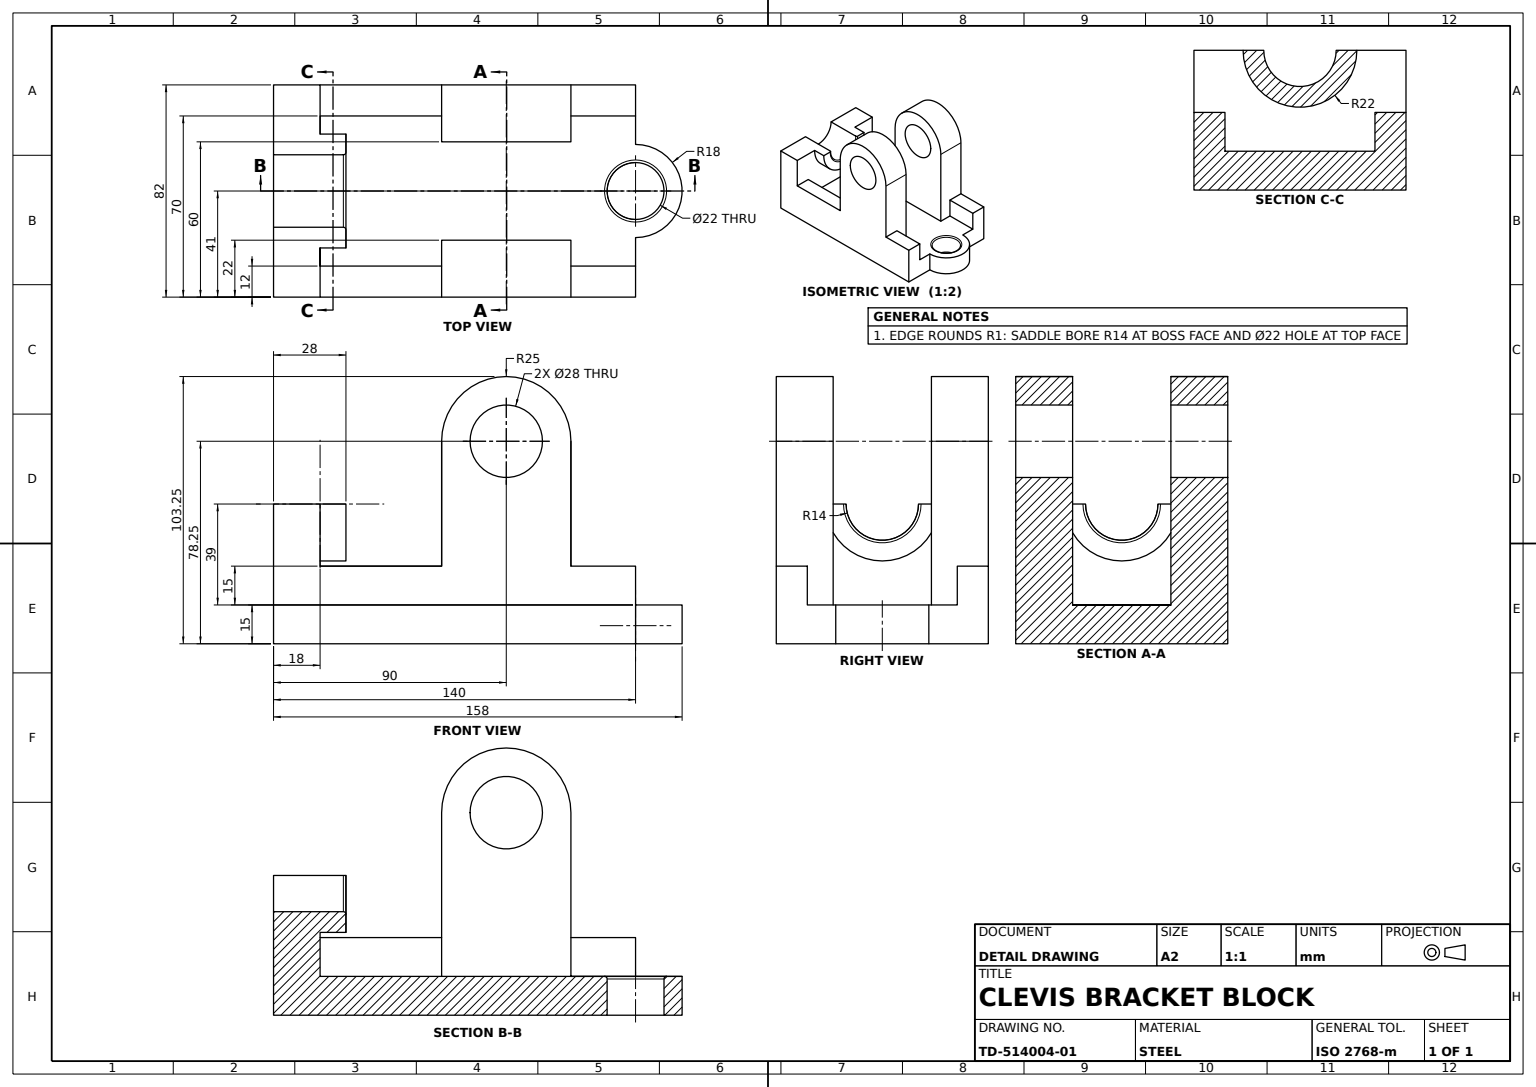
from build123d import *

# Parameters (mm, degrees)
BASE_PLATE_SKETCH_R     = 11
BASE_PLATE_DEPTH        = 15
REAR_WALL_SKETCH_W      = 18
REAR_WALL_SKETCH_H      = 82
REAR_WALL_DEPTH         = 39
STEP_BLOCKS_SKETCH_W    = 122
STEP_BLOCKS_SKETCH_H    = 12
STEP_BLOCKS_DEPTH       = 15
BEARING_EAR_1_SKETCH_R  = 14
BEARING_EAR_1_DEPTH     = 22
BEARING_START           = -22
BEARING_EAR_2_SKETCH_R  = 14
BEARING_EAR_2_DEPTH     = 22
SADDLE_CUT_DEPTH        = 22
SADDLE_BOSS_DEPTH       = 28
SADDLE_BOSS_FILLET_R1_R = 1
BASE_EDGE_FILLET_R1_R   = 1


with BuildPart() as part:
    # Base Plate Sketch → Base Plate (new body)
    with BuildSketch(Plane(origin=(0, 0, 0), x_dir=(1, 0, 0), z_dir=(0, 1, 0))):
        with BuildLine():
            Line((70, -18), (70, -41))
            Line((70, -41), (-70, -41))
            Line((-70, -41), (-70, 41))
            Line((-70, 41), (70, 41))
            Line((70, 41), (70, 18))
            ThreePointArc((70, 18), (88, 0), (70, -18))
        make_face()
        with Locations(Location((70, 0, 0), (0, 0, 270))):
            Circle(BASE_PLATE_SKETCH_R, mode=Mode.SUBTRACT)
    extrude(amount=BASE_PLATE_DEPTH)

    # Rear Wall Sketch → Rear Wall (add)
    with BuildSketch(Plane(origin=(0, 15, 0), x_dir=(1, 0, 0), z_dir=(0, 1, 0))):
        with Locations((-61, 0)):
            Rectangle(REAR_WALL_SKETCH_W, REAR_WALL_SKETCH_H)
    extrude(amount=REAR_WALL_DEPTH)

    # Step Blocks Sketch → Step Blocks (add)
    with BuildSketch(Plane(origin=(0, 15, 0), x_dir=(1, 0, 0), z_dir=(0, 1, 0))):
        with Locations((9, 35)):
            Rectangle(STEP_BLOCKS_SKETCH_W, STEP_BLOCKS_SKETCH_H)
        with Locations((9, -35)):
            Rectangle(STEP_BLOCKS_SKETCH_W, STEP_BLOCKS_SKETCH_H)
    extrude(amount=STEP_BLOCKS_DEPTH)

    # Bearing Ear 1 Sketch → Bearing Ear 1 (add)
    with BuildSketch(Plane.XY.offset(41)):
        with BuildLine():
            Line((-5, 78.254792273), (-5, 30))
            Line((-5, 30), (-5, 0))
            Line((-5, 0), (45, 0))
            Line((45, 0), (45, 30))
            Line((45, 30), (45, 78.254792273))
            ThreePointArc((45, 78.254792273), (20, 103.254792273), (-5, 78.254792273))
        make_face()
        with Locations((20, 78.254792273)):
            Circle(BEARING_EAR_1_SKETCH_R, mode=Mode.SUBTRACT)
    extrude(amount=-BEARING_EAR_1_DEPTH)

    # Bearing Ear 2 Sketch → Bearing Ear 2 (add)
    with BuildSketch(Plane(origin=(0, 0, -41), x_dir=(-1, 0, 0), z_dir=(0, 0, -1)).offset(BEARING_START)):
        with BuildLine():
            Line((-45, 78.254792273), (-45, 0))
            Line((-45, 0), (5, 0))
            Line((5, 0), (5, 78.254792273))
            ThreePointArc((5, 78.254792273), (-20, 103.254792273), (-45, 78.254792273))
        make_face()
        with Locations(Location((-20, 78.254792273, 0), (0, 0, 180))):
            Circle(BEARING_EAR_2_SKETCH_R, mode=Mode.SUBTRACT)
    extrude(amount=BEARING_EAR_2_DEPTH)

    # Saddle Cut Sketch → Saddle Cut (cut)
    with BuildSketch(Plane.ZY.offset(70)):
        with BuildLine():
            Line((-14, 54), (14, 54))
            ThreePointArc((14, 54), (0, 40), (-14, 54))
        make_face()
    extrude(amount=-SADDLE_CUT_DEPTH, mode=Mode.SUBTRACT)

    # Saddle Boss Sketch → Saddle Boss (add)
    with BuildSketch(Plane.ZY.offset(70)):
        with BuildLine():
            Line((-14, 54), (-22, 54))
            ThreePointArc((-22, 54), (0, 32), (22, 54))
            Line((22, 54), (14, 54))
            ThreePointArc((14, 54), (0, 40), (-14, 54))
        make_face()
    extrude(amount=-SADDLE_BOSS_DEPTH)

    # Saddle Boss Fillet R1
    saddle_boss_fillet_r1_edges = [part.edges().sort_by_distance(p)[0] for p in [
        (-42, 40, 0),
    ]]
    fillet(saddle_boss_fillet_r1_edges, radius=SADDLE_BOSS_FILLET_R1_R)

    # Base Edge Fillet R1
    base_edge_fillet_r1_edges = [part.edges().sort_by_distance(p)[0] for p in [
        (70, 15, -11),
    ]]
    fillet(base_edge_fillet_r1_edges, radius=BASE_EDGE_FILLET_R1_R)


solid = part.part
